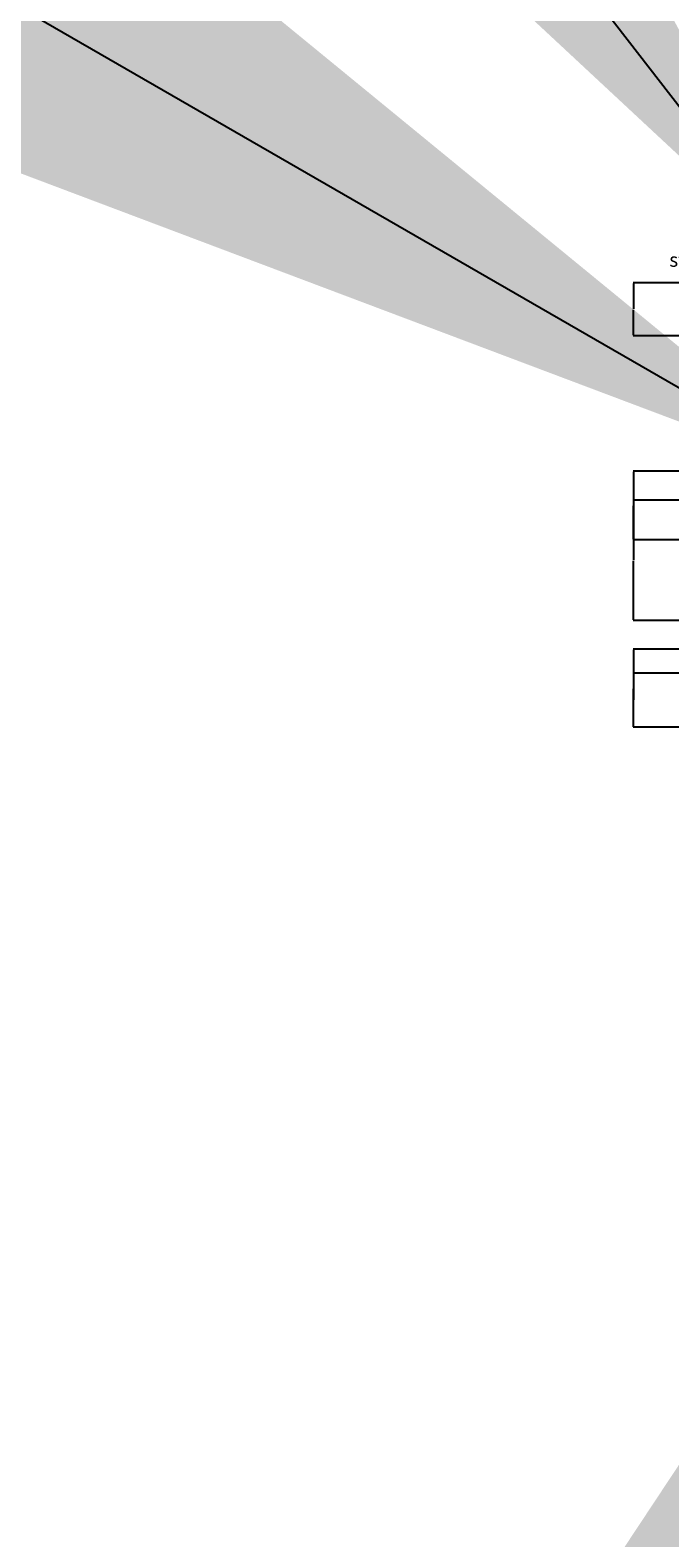
# Model space of a CAD drawing. Units: inches. Extents: x -9413 to 9703, y -9719 to 9096.
# Tile 1 of 1: x -249.7 to -0.3, y -311.2 to 276.8. Entities that reach past the tile are written whole.
import ezdxf
from ezdxf import colors
from ezdxf.entities.mleader import LeaderData, LeaderLine
from ezdxf.math import Vec2, Vec3

# ---------------------------------------------------------------- set-up
doc = ezdxf.new("R2010")
doc.units = ezdxf.units.IN
doc.header["$MEASUREMENT"] = 0
doc.layers.add('M-ANNO-TEXT', color=7, linetype='Continuous', lineweight=18)
doc.layers.add('M-DIMS', color=2, linetype='Continuous', lineweight=18)
doc.styles.get("Standard").update_dxf_attribs({"font": 'arial.ttf'})
doc.dimstyles.get("Standard").update_dxf_attribs({"dimtxt": 0.18, "dimasz": 0.18, "dimexe": 0.18, "dimexo": 0.0625, "dimgap": 0.09, "dimtad": 0, "dimtih": 1, "dimtoh": 1, "dimdec": 4, "dimzin": 0, "dimdsep": 46, "dimtxsty": 'Standard', "dimcen": 0.09, "dimadec": 0, "dimazin": 0, "dimtfac": 1, "dimtdec": 4, "dimtofl": 0, "dimtmove": 0, "dimatfit": 3, "dimfxl": 1, "dimtolj": 1, "dimtzin": 0, "dimarcsym": 0})

# ---------------------------------------------------------------- blocks, each defined once
blk = doc.blocks.new('*D7')
at = {"layer": 'Defpoints', "color": 0, "transparency": 16777216}
for p in [(-14.47089000000002, 35.36125100000002), (15.22950700000001, 35.36125100000002), (21.22715900000001, 4.961023000000001)]:
    blk.add_point(p, dxfattribs=at)
at = {"layer": 'M-DIMS', "color": 0, "lineweight": -2, "transparency": 16777216}
for p, q in [((15.16700700000001, 35.36125100000002), (-14.65089000000001, 35.36125100000002)), ((-14.47089000000002, 35.18125100000002), (-14.47089000000001, 20.34310152933151)), ((-14.47089000000001, 5.141022999999995), (-14.47089000000001, 19.97917247066849)), ((21.16465900000001, 4.961023000000001), (-14.65089000000001, 4.961022999999995))]:
    blk.add_line(p, q, dxfattribs=at)
at = {"layer": 'M-DIMS', "color": 0, "transparency": 16777216}
for points in [[(-14.50089000000001, 35.18125100000002), (-14.44089000000001, 35.18125100000002), (-14.47089000000002, 35.36125100000002)], [(-14.50089000000001, 5.141022999999995), (-14.44089000000001, 5.141022999999995), (-14.47089000000001, 4.961022999999995)]]:
    blk.add_solid(points, dxfattribs=at)
at = {"layer": 'M-DIMS', "color": 0, "transparency": 16777216, "insert": (-14.47089, 20.161137), "char_height": 0.18, "attachment_point": 5}
blk.add_mtext('\\A1;30.4', dxfattribs=at)
blk = doc.blocks.new('*D8')
at = {"layer": 'Defpoints', "color": 0, "transparency": 16777216}
for p in [(-14.47089000000002, 93.50315200000001), (69.11352000000002, 93.50315200000001), (69.11352000000002, 46.59639500000001)]:
    blk.add_point(p, dxfattribs=at)
at = {"layer": 'M-DIMS', "color": 0, "lineweight": -2, "transparency": 16777216}
for p, q in [((69.05102000000002, 93.50315200000001), (-14.65089000000003, 93.50315200000001)), ((-14.47089000000002, 93.32315200000001), (-14.47089000000001, 70.23167663778992)), ((-14.47089000000001, 46.776395), (-14.47089000000001, 69.86787036221011)), ((69.05102000000002, 46.59639500000001), (-14.65089000000002, 46.596395))]:
    blk.add_line(p, q, dxfattribs=at)
at = {"layer": 'M-DIMS', "color": 0, "transparency": 16777216}
for points in [[(-14.50089000000002, 93.32315200000001), (-14.44089000000002, 93.32315200000001), (-14.47089000000002, 93.50315200000001)], [(-14.50089000000001, 46.776395), (-14.44089000000001, 46.776395), (-14.47089000000001, 46.596395)]]:
    blk.add_solid(points, dxfattribs=at)
at = {"layer": 'M-DIMS', "color": 0, "transparency": 16777216, "insert": (-14.47088999999999, 70.0497735), "char_height": 0.18, "attachment_point": 5}
blk.add_mtext('\\A1;46.91', dxfattribs=at)
blk = doc.blocks.new('*D9')
at = {"layer": 'Defpoints', "color": 0, "transparency": 16777216}
for p in [(-14.47089000000002, 178.191776), (25.67423200000002, 178.191776), (42.03736800000001, 157.648001)]:
    blk.add_point(p, dxfattribs=at)
at = {"layer": 'M-DIMS', "color": 0, "lineweight": -2, "transparency": 16777216}
for p, q in [((25.61173200000002, 178.191776), (-14.65089000000002, 178.191776)), ((-14.47089000000002, 178.011776), (-14.47089000000001, 168.1017916377899)), ((-14.47089000000001, 157.828001), (-14.47089000000001, 167.7379853622101)), ((41.97486800000001, 157.648001), (-14.65089000000001, 157.648001))]:
    blk.add_line(p, q, dxfattribs=at)
at = {"layer": 'M-DIMS', "color": 0, "transparency": 16777216}
for points in [[(-14.50089000000001, 178.011776), (-14.44089000000001, 178.011776), (-14.47089000000002, 178.191776)], [(-14.50089000000001, 157.828001), (-14.44089000000001, 157.828001), (-14.47089000000001, 157.648001)]]:
    blk.add_solid(points, dxfattribs=at)
at = {"layer": 'M-DIMS', "color": 0, "transparency": 16777216, "insert": (-14.47088999999996, 167.9198885), "char_height": 0.18, "attachment_point": 5}
blk.add_mtext('\\A1;20.544', dxfattribs=at)
blk = doc.blocks.new('*D13')
at = {"layer": 'Defpoints', "color": 0, "transparency": 16777216}
for p in [(-14.47089000000002, 104.790816), (234.0943920000001, 104.790816), (234.0943920000001, 78.04556900000003)]:
    blk.add_point(p, dxfattribs=at)
at = {"layer": 'M-DIMS', "color": 0, "lineweight": -2, "transparency": 16777216}
for p, q in [((234.0318920000001, 104.790816), (-14.65089000000003, 104.790816)), ((-14.47089000000002, 104.610816), (-14.47089000000001, 91.6000956377899)), ((-14.47089000000001, 78.225569), (-14.47089000000001, 91.23628936221009)), ((234.0318920000001, 78.04556900000003), (-14.65089000000002, 78.04556899999999))]:
    blk.add_line(p, q, dxfattribs=at)
at = {"layer": 'M-DIMS', "color": 0, "transparency": 16777216}
for points in [[(-14.50089000000002, 104.610816), (-14.44089000000002, 104.610816), (-14.47089000000002, 104.790816)], [(-14.50089000000001, 78.225569), (-14.44089000000001, 78.225569), (-14.47089000000001, 78.04556899999999)]]:
    blk.add_solid(points, dxfattribs=at)
at = {"layer": 'M-DIMS', "color": 0, "transparency": 16777216, "insert": (-14.47088999999999, 91.41819249999998), "char_height": 0.18, "attachment_point": 5}
blk.add_mtext('\\A1;26.745', dxfattribs=at)
blk = doc.blocks.new('*D17')
at = {"layer": 'Defpoints', "color": 0, "transparency": 16777216}
for p in [(92.51182700000003, 26.01294900000001), (-14.47089000000001, 4.961022999999995), (21.22715900000001, 4.961023000000001)]:
    blk.add_point(p, dxfattribs=at)
at = {"layer": 'M-DIMS', "color": 0, "lineweight": -2, "transparency": 16777216}
for p, q in [((92.44932700000003, 26.01294900000001), (-14.65089000000002, 26.012949)), ((-14.47089000000002, 25.832949), (-14.47089000000001, 15.6688891377899)), ((-14.47089000000001, 5.141022999999995), (-14.47089000000001, 15.30508286221009)), ((21.16465900000001, 4.961023000000001), (-14.65089000000001, 4.961022999999995))]:
    blk.add_line(p, q, dxfattribs=at)
at = {"layer": 'M-DIMS', "color": 0, "transparency": 16777216}
for points in [[(-14.50089000000001, 25.832949), (-14.44089000000001, 25.832949), (-14.47089000000002, 26.012949)], [(-14.50089000000001, 5.141022999999995), (-14.44089000000001, 5.141022999999995), (-14.47089000000001, 4.961022999999995)]]:
    blk.add_solid(points, dxfattribs=at)
at = {"layer": 'M-DIMS', "color": 0, "transparency": 16777216, "insert": (-14.47089, 15.48698599999999), "char_height": 0.18, "attachment_point": 5}
blk.add_mtext('\\A1;21.05', dxfattribs=at)

msp = doc.modelspace()

# ---------------------------------------------------------------- dimensions: what is measured, and where the dimension line sits
at = {"layer": 'M-DIMS'}
for base, p1, p2, override, picture, middle in [((-14.47089000000002, 178.191776), (42.037368, 157.648001), (25.674232, 178.191776), {"dimdec": 3, "dimlfac": 1, "dimrnd": 0, "dimzin": 0, "dimdsep": 46, "dimlunit": 2}, '*D9', (-14.47088999999996, 167.9198885)), ((-14.47089000000002, 104.790816), (234.094392, 78.045569), (234.094392, 104.790816), {"dimdec": 3, "dimlfac": 1, "dimrnd": 0, "dimzin": 0, "dimdsep": 46, "dimlunit": 2}, '*D13', (-14.47088999999999, 91.41819249999998)), ((-14.47089000000002, 93.50315200000001), (69.11352, 46.59639499999999), (69.11352, 93.503152), {"dimdec": 2, "dimlfac": 1, "dimrnd": 0, "dimzin": 0, "dimdsep": 46, "dimlunit": 2}, '*D8', (-14.47088999999999, 70.0497735)), ((-14.47089000000002, 35.36125100000002), (21.227159, 4.961022999999999), (15.229507, 35.361251), {"dimdec": 1, "dimlfac": 1, "dimrnd": 0, "dimzin": 0, "dimdsep": 46, "dimlunit": 2}, '*D7', (-14.47089, 20.161137)), ((-14.47089000000001, 4.961022999999995), (92.511827, 26.012949), (21.227159, 4.961022999999999), {"dimdec": 2, "dimlfac": 1, "dimrnd": 0, "dimzin": 0, "dimdsep": 46, "dimlunit": 2}, '*D17', (-14.47089, 15.48698599999999))]:
    dim = msp.add_linear_dim(base=base, p1=p1, p2=p2, angle=90, dimstyle='Standard', override=override, dxfattribs=at)
    dim.commit()
    dim.dimension.update_dxf_attribs({"geometry": picture, "text_midpoint": middle})

# ---------------------------------------------------------------- leaders
at = {"layer": 'M-ANNO-TEXT'}
ml = msp.add_multileader_mtext('Standard', dxfattribs=at)
ml.set_content('steam drum', color=256)
ml.set_leader_properties()
ml.build(insert=Vec2(0, 0))
ml.multileader.update_dxf_attribs({"dogleg_length": 0.36, "arrow_head_size": 10000, "scale": 10})
ctx = ml.context
ctx.base_point, ctx.scale, ctx.char_height, ctx.arrow_head_size, ctx.landing_gap_size, ctx.plane_origin = Vec3(1.078100315116472, 187.1657656808087), 10, 5.4, 10000, 0.9, Vec3(56.53630785249729, 178.1917761520126)
ctx.text_align_type = 2
notes = []
notes.append((ctx, [(0, (1, 1, 0), (49.60206616053652, 187.1657656808087), (-1, 0), 7.616326009130828, [(0, [(56.5363078524973, 178.1917761520126)], 0, [])])]))
ctx.mtext.insert, ctx.mtext.alignment, ctx.mtext.flow_direction = Vec3(41.08574015140569, 189.9099675907678), 3, 5
ml = msp.add_multileader_mtext('Standard', dxfattribs=at)
ml.set_content('Boiler', color=256)
ml.set_leader_properties()
ml.build(insert=Vec2(0, 0))
ml.multileader.update_dxf_attribs({"dogleg_length": 0.36, "arrow_head_size": 10000, "scale": 10})
ctx = ml.context
ctx.base_point, ctx.scale, ctx.char_height, ctx.arrow_head_size, ctx.landing_gap_size, ctx.plane_origin = Vec3(31.04430257849453, 103.0991380116177), 10, 5.4, 10000, 0.9, Vec3(69.11352005531556, 99.3051261342938)
ctx.text_align_type = 2
notes.append((ctx, [(0, (1, 1, 0), (62.54209871927075, 103.0991380116177), (-1, 0), 10.86041551321825, [(0, [(69.11352005531556, 99.3051261342938)], 0, [])])]))
ctx.mtext.insert, ctx.mtext.alignment, ctx.mtext.flow_direction = Vec3(50.7816832060525, 105.8433399215768), 3, 5
ml = msp.add_multileader_mtext('Standard', dxfattribs=at)
ml.set_content('Air preheater', color=256)
ml.set_leader_properties()
ml.build(insert=Vec2(0, 0))
ml.multileader.update_dxf_attribs({"dogleg_length": 0.36, "arrow_head_size": 10000, "scale": 10})
ctx = ml.context
ctx.base_point, ctx.scale, ctx.char_height, ctx.arrow_head_size, ctx.landing_gap_size, ctx.plane_origin = Vec3(229.7079293124727, 37.30650895205824), 10, 5.4, 10000, 0.9, Vec3(241.9833706008503, 78.04556948044049)
notes.append((ctx, [(1, (1, 1, 0), (223.7048975654645, 37.30650895205824), (1, 0), 6.003031747008185, [(0, [(241.9833706008503, 78.04556948044049)], 0, [])])]))
ctx.mtext.insert, ctx.mtext.flow_direction = Vec3(230.6079293124727, 40.75609967511417), 5
for ctx, leaders in notes:
    for number, flags, end, landing, length, lines in leaders:
        leader = LeaderData()
        leader.index, (leader.has_last_leader_line, leader.has_dogleg_vector, leader.attachment_direction) = number, flags
        leader.last_leader_point, leader.dogleg_vector, leader.dogleg_length = Vec3(end), Vec3(landing), length
        for number, points, colour, breaks in lines:
            line = LeaderLine()
            line.index, line.vertices, line.color, line.breaks = number, Vec3.list(points), colors.encode_raw_color(colour), breaks
            leader.lines.append(line)
        ctx.leaders.append(leader)

doc.saveas('drawing.dxf')
